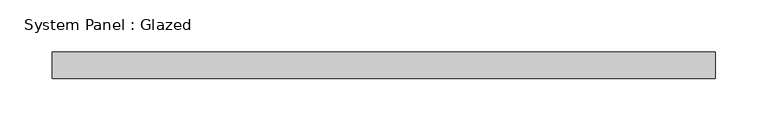
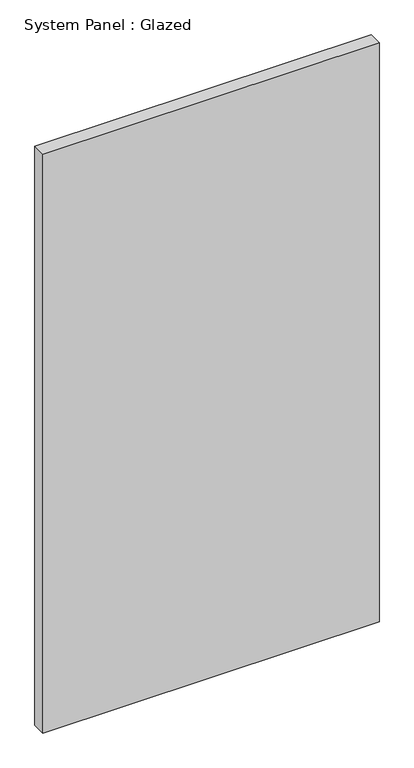
"""IFC4 building model written with IfcOpenShell, lengths in millimetres: plate geometry, System Panel : Glazed."""

from ifc_helpers import new_model, si_unit, origin, origin_with_axes, place, context, project, spatial, polyline, outline, extrude, source, transform, mapped, element, save


def system_panel_glazed_6a65e850(model_context):
    return source(origin(), model_context, "Body", "SweptSolid", [
        extrude(outline(polyline([(317.5, 19.05), (-317.5, 19.05), (-317.5, 44.45), (317.5, 44.45), (317.5, 19.05)])), origin_with_axes(), (0.0, 0.0, 1.0), 1155.7),
    ])


if __name__ == "__main__":
    model = new_model("IFC4")
    model_context = context("Model", 3, world=origin())
    ifc_project = project(units=[si_unit("LENGTHUNIT", "METRE", prefix="MILLI")], contexts=[model_context])
    site = spatial("IfcSite", under=ifc_project)
    building = spatial("IfcBuilding", under=site)
    placement = place(None, origin())
    system_panel_glazed_shape = system_panel_glazed_6a65e850(model_context)
    element("IfcPlate", 1, ObjectType="System Panel : Glazed", at=placement, inside=building, context=model_context, shape_type="MappedRepresentation", body=[
        mapped(system_panel_glazed_shape, transform((0.0, 0.0, 0.0), x_axis=(1.0, 0.0, 0.0), y_axis=(0.0, 1.0, 0.0), z_axis=(0.0, 0.0, 1.0))),
    ])
    save(model, "model.ifc")

# Revit data of these elements
# Type "System Panel : Glazed"
#   Construction Type Id = "GSP4R"
#   Analytic Construction = "1/8 in Pilkington single glazing"
#   Visual Light Transmittance = 0.9
#   Solar Heat Gain Coefficient = 0.86
#   Heat Transfer Coefficient (U) = 1.18115 BTU/(h·ft²·°F)
# Element 1 (IfcPlate, "System Panel : Glazed")
#   Materials on its faces: "Glass"
# Materials
#   "Glass": class "Glass", colour RGB 0 128 192, transparency 0.75, Description = "Soda Lime Glass", Cost = 0
